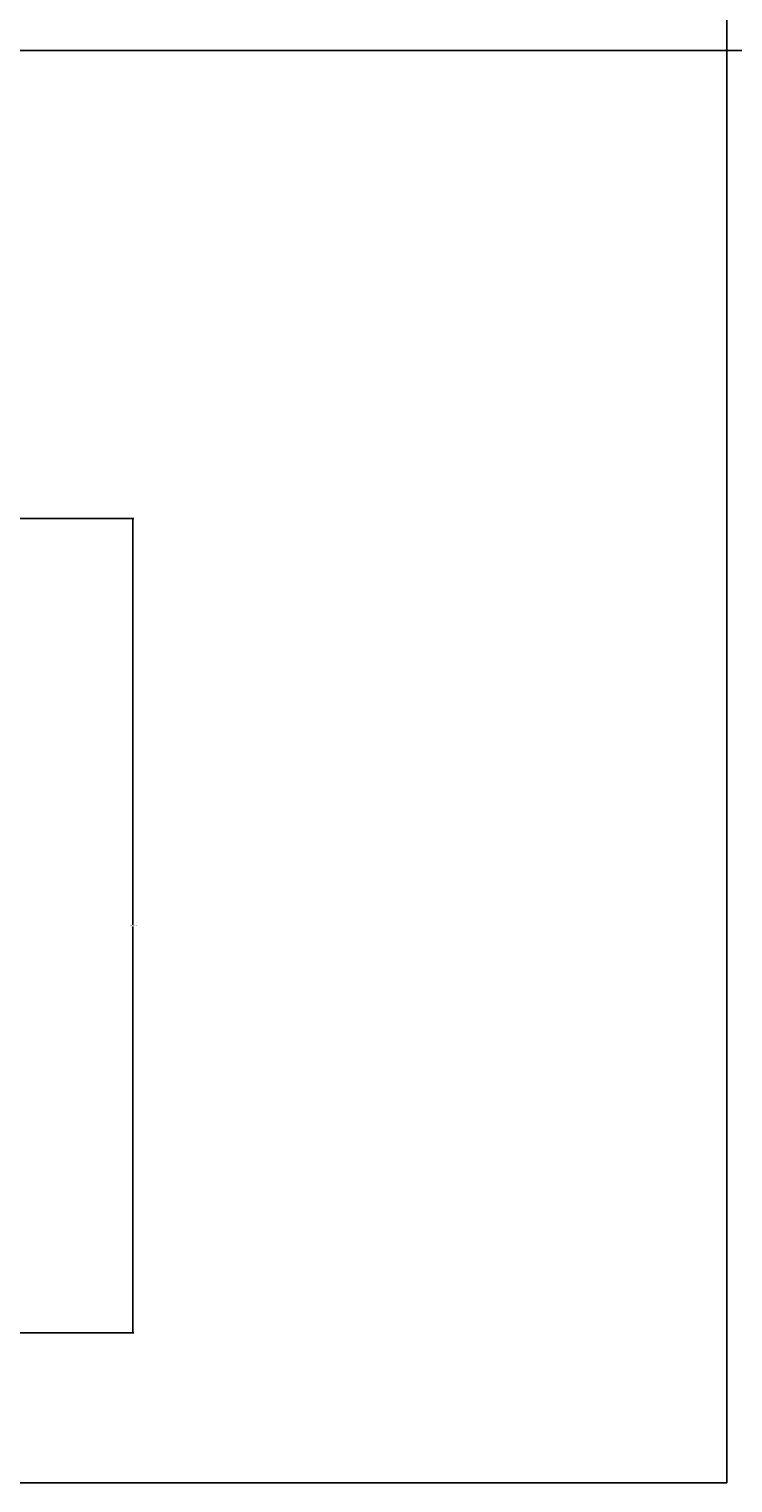
# Model space of a CAD drawing. Units: inches. Extents: x 1770 to 2988, y 1161 to 3221.
# Tile 5 of 44: x 2663 to 2804, y 1324 to 1614. Entities that reach past the tile are written whole.
import ezdxf

# ---------------------------------------------------------------- set-up
doc = ezdxf.new("R2010")
doc.units = ezdxf.units.IN
doc.layers.add('A-ANNO-DIMS', color=2, linetype='Continuous', lineweight=18)
doc.layers.add('C-PROP', color=7, linetype='Continuous', lineweight=25)
doc.styles.get("Standard").update_dxf_attribs({"font": 'arial.ttf'})
doc.dimstyles.get("Standard").update_dxf_attribs({"dimtxt": 0.18, "dimasz": 0.18, "dimexe": 0.18, "dimexo": 0.0625, "dimgap": 0.09, "dimtad": 0, "dimtih": 1, "dimtoh": 1, "dimdec": 4, "dimzin": 0, "dimdsep": 46, "dimtxsty": 'Standard', "dimcen": 0.09, "dimadec": 0, "dimazin": 0, "dimtfac": 1, "dimtdec": 4, "dimtofl": 0, "dimtmove": 0, "dimatfit": 3, "dimfxl": 1, "dimtolj": 1, "dimtzin": 0, "dimarcsym": 0})

# ---------------------------------------------------------------- blocks, each defined once
blk = doc.blocks.new('*D50')
at = {"layer": 'A-ANNO-DIMS', "color": 0, "lineweight": -2, "transparency": 16777216}
for p, q in [((2659.16, 1516.52), (2683.72, 1516.52)), ((2683.54, 1516.34), (2683.54, 1435.22)), ((2683.54, 1353.73), (2683.54, 1434.85)), ((2659.16, 1353.55), (2683.72, 1353.55))]:
    blk.add_line(p, q, dxfattribs=at)
at = {"layer": 'A-ANNO-DIMS', "color": 0, "transparency": 16777216}
for points in [[(2683.51, 1516.34), (2683.57, 1516.34), (2683.54, 1516.52)], [(2683.51, 1353.73), (2683.57, 1353.73), (2683.54, 1353.55)]]:
    blk.add_solid(points, dxfattribs=at)
at = {"layer": 'Defpoints', "color": 0, "transparency": 16777216}
for p in [(2659.1, 1516.52), (2683.54, 1516.52), (2659.1, 1353.55)]:
    blk.add_point(p, dxfattribs=at)
at = {"layer": 'A-ANNO-DIMS', "color": 0, "transparency": 16777216, "insert": (2683.54, 1435.04), "char_height": 0.18, "attachment_point": 5}
blk.add_mtext('\\A1;SEDAN 163 TYP.', dxfattribs=at)
blk = doc.blocks.new('*D61')
at = {"layer": 'A-ANNO-DIMS', "color": 0, "lineweight": -2, "transparency": 16777216}
for p, q in [((2625.76, 2376.7), (2866.87, 2376.7)), ((2866.69, 2376.52), (2866.69, 1993.63)), ((2866.69, 1610.38), (2866.69, 1993.27)), ((2625.76, 1610.2), (2866.87, 1610.2))]:
    blk.add_line(p, q, dxfattribs=at)
at = {"layer": 'A-ANNO-DIMS', "color": 0, "transparency": 16777216}
for points in [[(2866.66, 2376.52), (2866.72, 2376.52), (2866.69, 2376.7)], [(2866.66, 1610.38), (2866.72, 1610.38), (2866.69, 1610.2)]]:
    blk.add_solid(points, dxfattribs=at)
at = {"layer": 'Defpoints', "color": 0, "transparency": 16777216}
for p in [(2625.7, 2376.7), (2866.69, 2376.7), (2625.7, 1610.2)]:
    blk.add_point(p, dxfattribs=at)
at = {"layer": 'A-ANNO-DIMS', "color": 0, "transparency": 16777216, "insert": (2866.69, 1993.45), "char_height": 0.18, "attachment_point": 5}
blk.add_mtext('\\A1;766.5', dxfattribs=at)

msp = doc.modelspace()

# ---------------------------------------------------------------- linework, layer by layer
at = {"layer": 'C-PROP'}
msp.add_lwpolyline([(1971.5344, 2506.2747), (2802.4374, 2506.2747), (2802.4374, 1323.5288), (1971.5344, 1323.5288)], close=True, dxfattribs=at)

# ---------------------------------------------------------------- dimensions: what is measured, and where the dimension line sits
at = {"layer": 'A-ANNO-DIMS'}
dim = msp.add_linear_dim(base=(2866.6874, 2376.7021), p1=(2625.696, 1610.2021), p2=(2625.696, 2376.7021), angle=90, dimstyle='Standard', override={"dimdec": 1, "dimlfac": 1, "dimrnd": 0, "dimzin": 0, "dimdsep": 46, "dimlunit": 2}, dxfattribs=at)
dim.commit()
dim.dimension.update_dxf_attribs({"geometry": '*D61', "text_midpoint": (2866.6874, 1993.4521)})
dim = msp.add_linear_dim(base=(2683.5444, 1516.5237), p1=(2659.0986, 1353.5515), p2=(2659.0986, 1516.5237), angle=90, text='SEDAN <> TYP.', dimstyle='Standard', override={"dimdec": 0, "dimlfac": 1, "dimrnd": 0, "dimzin": 0, "dimdsep": 46, "dimlunit": 2}, dxfattribs=at)
dim.commit()
dim.dimension.update_dxf_attribs({"geometry": '*D50', "text_midpoint": (2683.5444, 1435.0376)})

doc.saveas('drawing.dxf')
